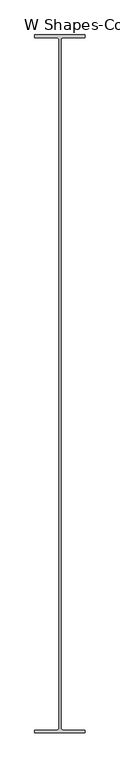
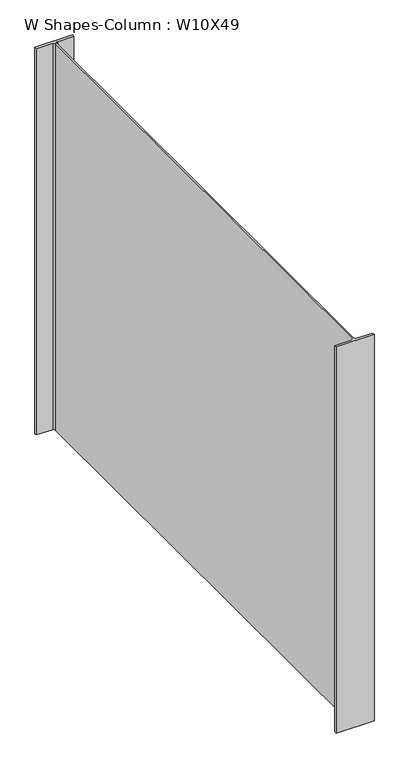
"""IFC4 building model written with IfcOpenShell, lengths in millimetres: column geometry, W Shapes-Column : W10X49."""

from ifc_helpers import new_model, si_unit, point, frame_2d, origin, origin_with_axes, place, context, project, spatial, polyline, circle_curve, trimmed, segment, composite_curve, outline, extrude, source, transform, mapped, element, save


def w_shapes_column_w10x49_8dea7e6f(model_context):
    return source(origin(), model_context, "Body", "SweptSolid", [
        extrude(outline(composite_curve([segment(polyline([(127.0, 1752.6), (127.0, 1738.376), (17.018, 1738.376)]), True, "CONTINUOUS"), segment(trimmed(circle_curve(frame_2d((17.018, 1725.676)), 12.7), [point((17.018, 1738.376))], [point((4.318, 1725.676))], True, "CARTESIAN"), True, "CONTINUOUS"), segment(polyline([(4.318, 1725.676), (4.318, -1725.676)]), True, "CONTINUOUS"), segment(trimmed(circle_curve(frame_2d((17.018, -1725.676)), 12.7), [point((4.318, -1725.676))], [point((17.018, -1738.376))], True, "CARTESIAN"), True, "CONTINUOUS"), segment(polyline([(17.018, -1738.376), (127.0, -1738.376), (127.0, -1752.6), (-127.0, -1752.6), (-127.0, -1738.376), (-17.018, -1738.376)]), True, "CONTINUOUS"), segment(trimmed(circle_curve(frame_2d((-17.018, -1725.676)), 12.7), [point((-17.018, -1738.376))], [point((-4.318, -1725.676))], True, "CARTESIAN"), True, "CONTINUOUS"), segment(polyline([(-4.318, -1725.676), (-4.318, 1725.676)]), True, "CONTINUOUS"), segment(trimmed(circle_curve(frame_2d((-17.018, 1725.676)), 12.7), [point((-4.318, 1725.676))], [point((-17.018, 1738.376))], True, "CARTESIAN"), True, "CONTINUOUS"), segment(polyline([(-17.018, 1738.376), (-127.0, 1738.376), (-127.0, 1752.6), (127.0, 1752.6)]), True, "CONTINUOUS")], self_intersect=False)), origin_with_axes(), (0.0, 0.0, 1.0), 2743.2),
    ])


if __name__ == "__main__":
    model = new_model("IFC4")
    model_context = context("Model", 3, world=origin())
    ifc_project = project(units=[si_unit("LENGTHUNIT", "METRE", prefix="MILLI")], contexts=[model_context])
    site = spatial("IfcSite", under=ifc_project)
    building = spatial("IfcBuilding", under=site)
    placement = place(None, origin())
    w_shapes_column_w10x49_shape = w_shapes_column_w10x49_8dea7e6f(model_context)
    element("IfcColumn", 1, ObjectType="W Shapes-Column : W10X49", at=placement, inside=building, context=model_context, shape_type="MappedRepresentation", body=[
        mapped(w_shapes_column_w10x49_shape, transform((0.0, 0.0, 0.0), x_axis=(1.0, 0.0, 0.0), y_axis=(0.0, 1.0, 0.0), z_axis=(0.0, 0.0, 1.0))),
    ])
    save(model, "model.ifc")

# Revit data of these elements
# Type "W Shapes-Column : W10X49"
#   Section Name Key = "W10x49"
#   Assembly Code = "B10"
#   Width = 10.000"
#   Web Thickness = 0.340"
#   Web Fillet = 0.500"
#   Warping Constant = 2070.00 in⁶
#   Torsional Moment of Inertia = 1.39 in⁴
#   Section Area = 14.40 in²
#   Plastic Modulus weak axis = 28.30 in³
#   Plastic Modulus strong axis = 60.40 in³
#   Perimeter = 58.50 ft²/ft
#   Nominal Weight = 49.00 lbf/ft
#   Moment of Inertia weak axis = 93.40 in⁴
#   Moment of Inertia strong axis = 272.00 in⁴
#   Height = 138.000"
#   Flange Thickness = 0.560"
#   Elastic Modulus weak axis = 18.70 in³
#   Elastic Modulus strong axis = 54.60 in³
#   Centroid Vertical = 69.000"
#   Centroid Horizontal = 5.000"
#   Structural Material [instance default] = Steel ASTM A992
#   Principal Axes Angle = 0
# Element 1 (IfcColumn, "W Shapes-Column : W10X49")
#   Materials on its faces: "Steel ASTM A992"
# Materials
#   "Steel ASTM A992": class "Metal", colour RGB 199 199 199, transparency 0, Description = "Structural steel 50ksi", Cost = 0
